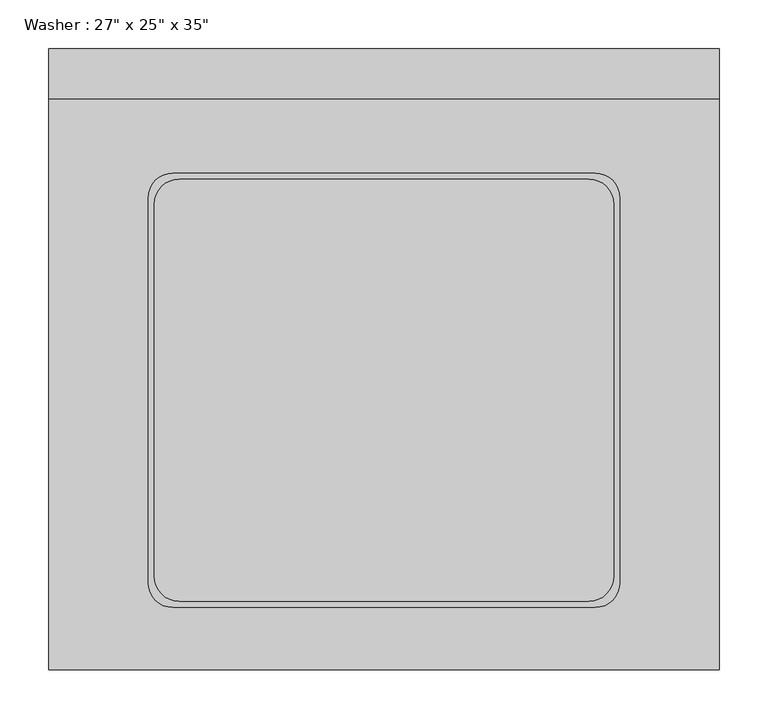
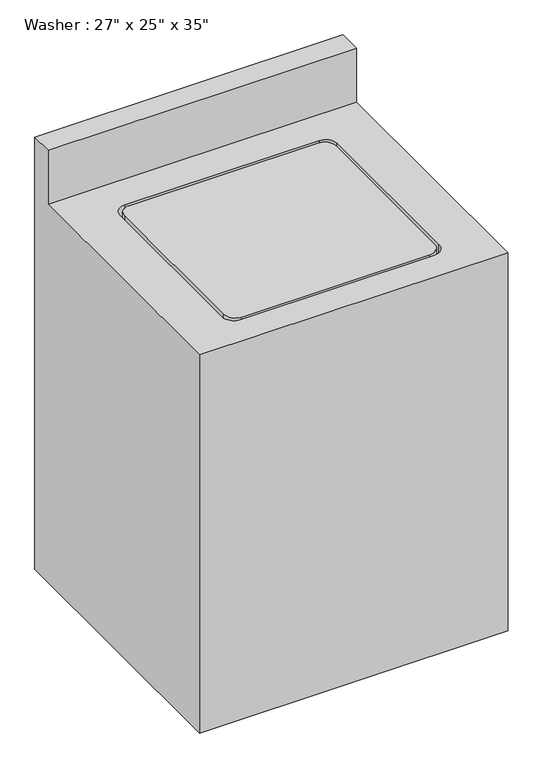
"""IFC4 building model written with IfcOpenShell, lengths in millimetres: proxy geometry."""

from ifc_helpers import new_model, si_unit, point, frame, frame_2d, origin, place, context, project, spatial, polyline, circle_curve, trimmed, segment, composite_curve, outline, extrude, source, transform, mapped, element, save
from ifc_brep_helpers import plane_surface, revolved_surface, advanced_brep


def proxy_718fa39f(model_context):
    return source(origin(), model_context, "Body", "SolidModel", [
        extrude(outline(composite_curve([segment(trimmed(circle_curve(frame_2d((210.8674685, 437.8995648)), 25.4), [point((185.4674685, 437.8995648))], [point((210.8674685, 463.2995648))], False, "CARTESIAN"), True, "CONTINUOUS"), segment(polyline([(210.8674685, 463.2995648), (629.9674685, 463.2995648)]), True, "CONTINUOUS"), segment(trimmed(circle_curve(frame_2d((629.9674685, 437.8995648)), 25.4), [point((629.9674685, 463.2995648))], [point((655.3674685, 437.8995648))], False, "CARTESIAN"), True, "CONTINUOUS"), segment(polyline([(655.3674685, 437.8995648), (655.3674685, 56.8995648)]), True, "CONTINUOUS"), segment(trimmed(circle_curve(frame_2d((629.9674685, 56.8995648)), 25.4), [point((655.3674685, 56.8995648))], [point((629.9674685, 31.4995648))], False, "CARTESIAN"), True, "CONTINUOUS"), segment(polyline([(629.9674685, 31.4995648), (210.8674685, 31.4995648)]), True, "CONTINUOUS"), segment(trimmed(circle_curve(frame_2d((210.8674685, 56.8995648)), 25.4), [point((210.8674685, 31.4995648))], [point((185.4674685, 56.8995648))], False, "CARTESIAN"), True, "CONTINUOUS"), segment(polyline([(185.4674685, 56.8995648), (185.4674685, 437.8995648)]), True, "CONTINUOUS")], self_intersect=False)), frame((0.0, 0.0, 863.6), z_axis=(0.0, 0.0, 1.0), x_axis=(1.0, 0.0, 0.0)), (0.0, 0.0, 1.0), 25.4),
        advanced_brep(
        [(77.5174685, 545.8495648, 889.0), (77.5174685, 545.8495648, 1016.0), (77.5174685, 596.6495648, 1016.0), (77.5174685, 596.6495648, 0.0), (77.5174685, -38.3504352, 0.0), (77.5174685, -38.3504352, 889.0), (763.3174685, 596.6495648, 1016.0), (763.3174685, 545.8495648, 1016.0), (763.3174685, 545.8495648, 889.0), (763.3174685, -38.3504352, 889.0), (763.3174685, -38.3504352, 0.0), (763.3174685, 596.6495648, 0.0), (204.5174685, 469.4681955, 889.0), (636.3174685, 469.4681955, 889.0), (661.7174685, 444.0681955, 889.0), (661.7174685, 50.5495648, 889.0), (636.3174685, 25.1495648, 889.0), (204.5174685, 25.1495648, 889.0), (179.1174685, 50.5495648, 889.0), (179.1174685, 444.0681955, 889.0), (636.3174685, 469.4681955, 838.2), (204.5174685, 469.4681955, 838.2), (179.1174685, 444.0681955, 838.2), (179.1174685, 50.5495648, 838.2), (204.5174685, 25.1495648, 838.2), (636.3174685, 25.1495648, 838.2), (661.7174685, 50.5495648, 838.2), (661.7174685, 444.0681955, 838.2)],
        [
            (0, 1),
            (1, 2),
            (2, 3),
            (3, 4),
            (4, 5),
            (5, 0),
            (6, 7),
            (7, 8),
            (8, 9),
            (9, 10),
            (10, 11),
            (11, 6),
            (0, 8),
            (7, 1),
            (6, 2),
            (11, 3),
            (5, 9),
            (12, 13),
            (13, 14, circle_curve(frame((636.3174685, 444.0681955, 889.0), z_axis=(0.0, 0.0, -1.0), x_axis=(0.0, -1.0, 0.0)), 25.4)),
            (14, 15),
            (15, 16, circle_curve(frame((636.3174685, 50.5495648, 889.0), z_axis=(0.0, 0.0, -1.0), x_axis=(0.0, -1.0, 0.0)), 25.4)),
            (16, 17),
            (17, 18, circle_curve(frame((204.5174685, 50.5495648, 889.0), z_axis=(0.0, 0.0, -1.0), x_axis=(0.0, -1.0, 0.0)), 25.4)),
            (18, 19),
            (19, 12, circle_curve(frame((204.5174685, 444.0681955, 889.0), z_axis=(0.0, 0.0, -1.0), x_axis=(0.0, -1.0, 0.0)), 25.4)),
            (10, 4),
            (20, 21),
            (21, 22, circle_curve(frame((204.5174685, 444.0681955, 838.2), z_axis=(0.0, 0.0, 1.0), x_axis=(0.0, -1.0, 0.0)), 25.4)),
            (22, 23),
            (23, 24, circle_curve(frame((204.5174685, 50.5495648, 838.2), z_axis=(0.0, 0.0, 1.0), x_axis=(0.0, -1.0, 0.0)), 25.4)),
            (24, 25),
            (25, 26, circle_curve(frame((636.3174685, 50.5495648, 838.2), z_axis=(0.0, 0.0, 1.0), x_axis=(0.0, -1.0, 0.0)), 25.4)),
            (26, 27),
            (27, 20, circle_curve(frame((636.3174685, 444.0681955, 838.2), z_axis=(0.0, 0.0, 1.0), x_axis=(0.0, -1.0, 0.0)), 25.4)),
            (20, 13),
            (12, 21),
            (19, 22),
            (18, 23),
            (17, 24),
            (16, 25),
            (15, 26),
            (14, 27),
        ],
        [
            plane_surface(frame((77.5174685, 545.8495648, 889.0), z_axis=(-1.0, 0.0, 0.0), x_axis=(0.0, 0.0, 1.0))),
            plane_surface(frame((763.3174685, 545.8495648, 889.0), z_axis=(1.0, 0.0, 0.0), x_axis=(0.0, 0.0, -1.0))),
            plane_surface(frame((77.5174685, 545.8495648, 889.0), z_axis=(0.0, -1.0, 0.0), x_axis=(1.0, 0.0, 0.0))),
            plane_surface(frame((77.5174685, 545.8495648, 1016.0), z_axis=(0.0, 0.0, 1.0), x_axis=(1.0, 0.0, 0.0))),
            plane_surface(frame((77.5174685, 596.6495648, 1016.0), z_axis=(0.0, 1.0, 0.0), x_axis=(1.0, 0.0, 0.0))),
            plane_surface(frame((77.5174685, -38.3504352, 889.0), z_axis=(0.0, 0.0, 1.0), x_axis=(0.0, -1.0, 0.0))),
            plane_surface(frame((77.5174685, -38.3504352, 0.0), z_axis=(0.0, 0.0, -1.0), x_axis=(0.0, 1.0, 0.0))),
            plane_surface(frame((77.5174685, -38.3504352, 889.0), z_axis=(0.0, -1.0, 0.0), x_axis=(0.0, 0.0, -1.0))),
            plane_surface(frame((204.5174685, 469.4681955, 838.2), z_axis=(0.0, 0.0, 1.0), x_axis=(1.0, 0.0, 0.0))),
            plane_surface(frame((636.3174685, 469.4681955, 889.0), z_axis=(0.0, -1.0, 0.0), x_axis=(0.0, 0.0, -1.0))),
            revolved_surface(polyline([(204.5174685, 418.6681955, 889.0), (204.5174685, 418.6681955, 838.2)]), (204.5174685, 444.0681955, 838.2), (0.0, 0.0, 1.0)),
            plane_surface(frame((179.1174685, 444.0681955, 889.0), z_axis=(1.0, 0.0, 0.0), x_axis=(0.0, 0.0, -1.0))),
            revolved_surface(polyline([(204.5174685, 25.1495648, 889.0), (204.5174685, 25.1495648, 838.2)]), (204.5174685, 50.5495648, 838.2), (0.0, 0.0, 1.0)),
            plane_surface(frame((204.5174685, 25.1495648, 889.0), z_axis=(0.0, 1.0, 0.0), x_axis=(0.0, 0.0, -1.0))),
            revolved_surface(polyline([(636.3174685, 25.1495648, 889.0), (636.3174685, 25.1495648, 838.2)]), (636.3174685, 50.5495648, 838.2), (0.0, 0.0, 1.0)),
            plane_surface(frame((661.7174685, 50.5495648, 889.0), z_axis=(-1.0, 0.0, 0.0), x_axis=(0.0, 0.0, -1.0))),
            revolved_surface(polyline([(636.3174685, 418.6681955, 889.0), (636.3174685, 418.6681955, 838.2)]), (636.3174685, 444.0681955, 838.2), (0.0, 0.0, 1.0)),
        ],
        [
            (0, [[1, 2, 3, 4, 5, 6]]),
            (1, [[7, 8, 9, 10, 11, 12]]),
            (2, [[-1, 13, -8, 14]]),
            (3, [[-2, -14, -7, 15]]),
            (4, [[-15, -12, 16, -3]]),
            (5, [[17, -9, -13, -6], [18, 19, 20, 21, 22, 23, 24, 25]]),
            (6, [[-16, -11, 26, -4]]),
            (7, [[-17, -5, -26, -10]]),
            (8, [[27, 28, 29, 30, 31, 32, 33, 34]]),
            (9, [[-27, 35, -18, 36]]),
            (10, [[-28, -36, -25, 37]]),
            (11, [[-29, -37, -24, 38]]),
            (12, [[-30, -38, -23, 39]]),
            (13, [[-31, -39, -22, 40]]),
            (14, [[-32, -40, -21, 41]]),
            (15, [[-33, -41, -20, 42]]),
            (16, [[-34, -42, -19, -35]]),
        ],
    ),
    ])


if __name__ == "__main__":
    model = new_model("IFC4")
    model_context = context("Model", 3, world=origin())
    ifc_project = project(units=[si_unit("LENGTHUNIT", "METRE", prefix="MILLI")], contexts=[model_context])
    site = spatial("IfcSite", under=ifc_project)
    building = spatial("IfcBuilding", under=site)
    placement = place(None, origin())
    proxy_shape = proxy_718fa39f(model_context)
    element("IfcBuildingElementProxy", 1, Name="Washer : 27\" x 25\" x 35\"", ObjectType="Washer : 27\" x 25\" x 35\"", at=placement, inside=building, context=model_context, shape_type="MappedRepresentation", body=[
        mapped(proxy_shape, transform((0.0, 0.0, 0.0), x_axis=(1.0, 0.0, 0.0), y_axis=(0.0, 1.0, 0.0), z_axis=(0.0, 0.0, 1.0))),
    ])
    save(model, "model.ifc")

# Revit data of these elements
# Type "Washer : 27\" x 25\" x 35\""
#   Label = "W"
#   Assembly Code = "E1090400"
#   Depth = 2' - 1"
#   Height = 2' - 11"
#   Width = 2' - 3"
#   Washer Material = Steel, Paint Finish, Ivory, Matte
#   Default Elevation = 0
# Element 1 (IfcBuildingElementProxy, "Washer : 27\" x 25\" x 35\"")
#   Materials on its faces: "Steel, Paint Finish, Ivory, Matte"
# Materials
#   "Steel, Paint Finish, Ivory, Matte": class "Metal", colour RGB 247 247 239, transparency 0, Description = "Steel, paint finish, ivory, matte", Cost = 0
